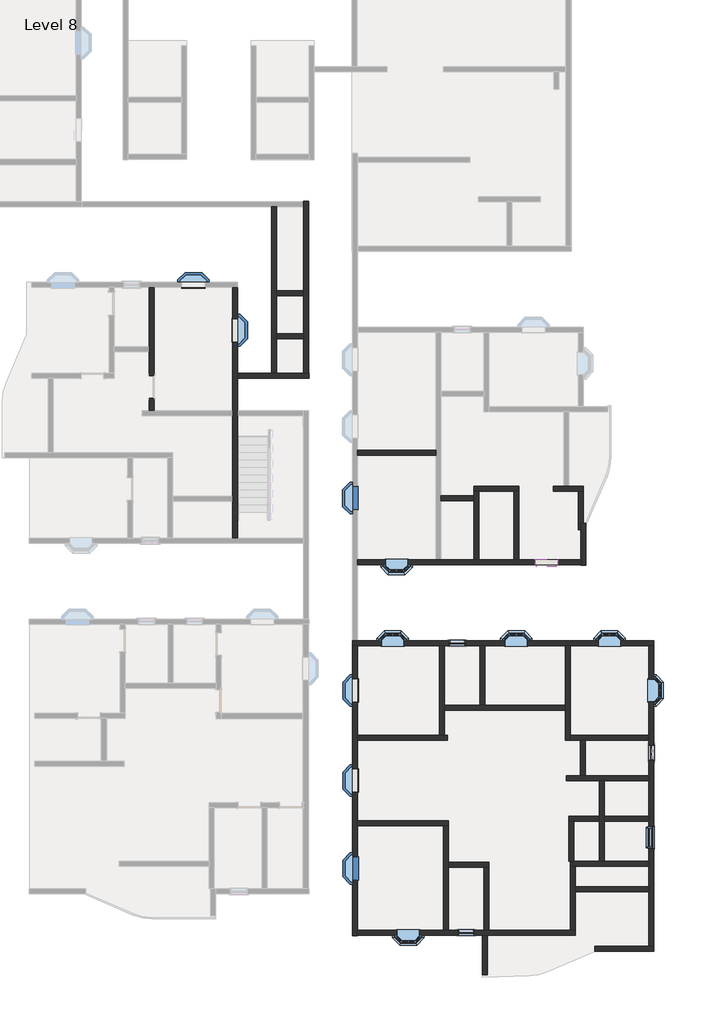
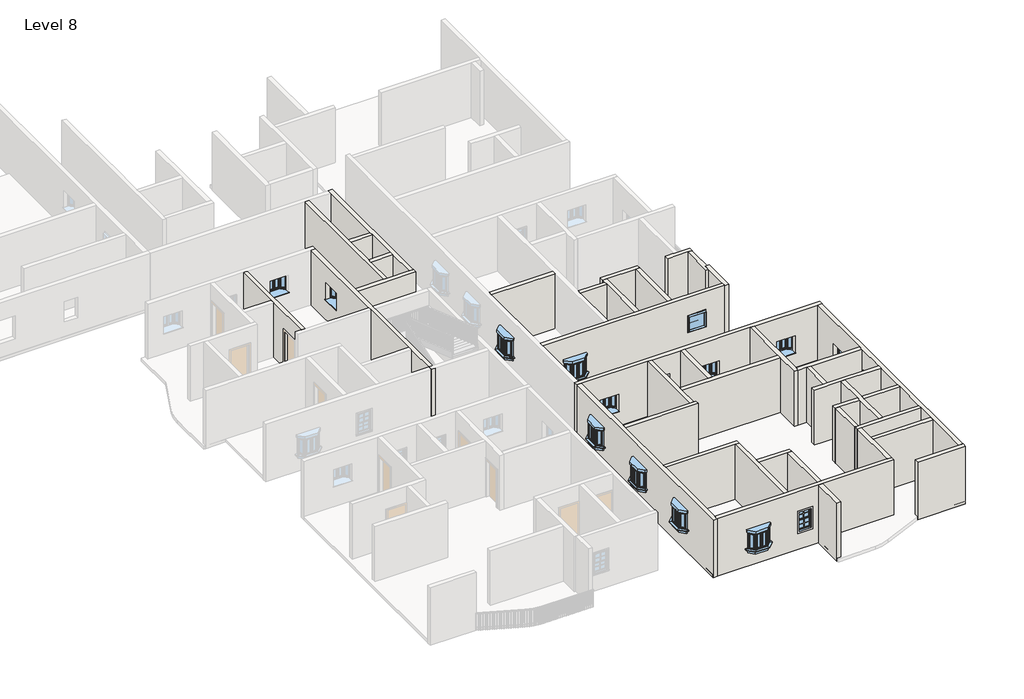
# One storey, part 2 of 14: 40 walls, 17 windows.
"""IFC4 building model written with IfcOpenShell, lengths in millimetres."""

from ifc_helpers import new_model, si_unit, frame, origin, place, context, project, spatial, polyline, outline, extrude, faceted_brep, transform, mapped, element, save
from components import window_910x910mm_67ef725a, window_8debb0fa, windows_sgl_w_glazing_bars_910x910mm_256712d0

model = new_model("IFC4")

# Units and contexts
model_context = context("Model", 3, world=origin())
ifc_project = project(units=[si_unit("LENGTHUNIT", "METRE", prefix="MILLI")], contexts=[model_context])

# Site, building, storey
site = spatial("IfcSite", under=ifc_project)
building = spatial("IfcBuilding", under=site)
storey = spatial("IfcBuildingStorey", under=building, Name="Level 8", Elevation=21336.0)

# Walls
placement = place(None, origin())
element("IfcWall", 1, ObjectType="4.5\" p", at=placement, inside=storey, context=model_context, shape_type="SweptSolid", body=[
    extrude(outline(polyline([(6070.4380523, -28382.7374148), (6070.4380523, -26796.6042694), (6273.6380523, -26796.6042694), (6273.6380523, -28382.7374148), (6070.4380523, -28382.7374148)])), frame((0.0, 0.0, 21336.0), z_axis=(0.0, 0.0, 1.0), x_axis=(1.0, 0.0, 0.0)), (0.0, 0.0, 1.0), 3048.0),
])
element("IfcWall", 2, ObjectType="4.5\" p", at=placement, inside=storey, context=model_context, shape_type="Brep", body=[
    faceted_brep([(10639.6896214, -27431.6042694, 21336.0), (13030.0380523, -27431.6042694, 21336.0), (13030.0380523, -27431.6042694, 24384.0), (10639.6896214, -27431.6042694, 24384.0), (10639.6896214, -27228.4042694, 21336.0), (10639.6896214, -27228.4042694, 24384.0), (12814.1380523, -27228.4042694, 24384.0), (13017.3380523, -27228.4042694, 24384.0), (13030.0380523, -27228.4042694, 24384.0), (13030.0380523, -27228.4042694, 21336.0), (13017.3380523, -27228.4042694, 21336.0), (12814.1380523, -27228.4042694, 21336.0)], [[[0, 1, 2, 3]], [[4, 5, 6, 7, 8, 9, 10, 11]], [[1, 0, 4, 11, 10, 9]], [[2, 1, 9, 8]], [[3, 2, 8, 7, 6, 5]], [[0, 3, 5, 4]]]),
])
element("IfcWall", 3, ObjectType="4.5\" p", at=placement, inside=storey, context=model_context, shape_type="Brep", body=[
    faceted_brep([(1015.8380523, -18878.1542694, 21336.0), (4648.0380523, -18878.1542694, 21336.0), (4648.0380523, -18878.1542694, 24384.0), (1015.8380523, -18878.1542694, 24384.0), (1015.8380523, -18674.9542694, 21336.0), (1015.8380523, -18674.9542694, 24384.0), (4336.8880523, -18674.9542694, 24384.0), (4540.0880523, -18674.9542694, 24384.0), (4648.0380523, -18674.9542694, 24384.0), (4648.0380523, -18674.9542694, 21336.0), (4540.0880523, -18674.9542694, 21336.0), (4336.8880523, -18674.9542694, 21336.0)], [[[0, 1, 2, 3]], [[4, 5, 6, 7, 8, 9, 10, 11]], [[1, 0, 4, 11, 10, 9]], [[2, 1, 9, 8]], [[3, 2, 8, 7, 6, 5]], [[0, 3, 5, 4]]]),
])
element("IfcWall", 4, ObjectType="4.5\" p", at=placement, inside=storey, context=model_context, shape_type="Brep", body=[
    faceted_brep([(4336.8880523, -15049.1042694, 21336.0), (4336.8880523, -18674.9542694, 21336.0), (4336.8880523, -18674.9542694, 24384.0), (4336.8880523, -15049.1042694, 24384.0), (4540.0880523, -15049.1042694, 21336.0), (4540.0880523, -15049.1042694, 24384.0), (4540.0880523, -17455.7542694, 24384.0), (4540.0880523, -17658.9542694, 24384.0), (4540.0880523, -18674.9542694, 24384.0), (4540.0880523, -18674.9542694, 21336.0), (4540.0880523, -17658.9542694, 21336.0), (4540.0880523, -17455.7542694, 21336.0)], [[[0, 1, 2, 3]], [[4, 5, 6, 7, 8, 9, 10, 11]], [[1, 0, 4, 11, 10, 9]], [[3, 2, 8, 7, 6, 5]], [[0, 3, 5, 4]], [[2, 1, 9, 8]]]),
])
element("IfcWall", 5, ObjectType="4.5\" p", at=placement, inside=storey, context=model_context, shape_type="Brep", body=[
    faceted_brep([(4540.0880523, -17658.9542694, 21336.0), (9442.2880523, -17658.9542694, 21336.0), (9442.2880523, -17658.9542694, 24384.0), (4540.0880523, -17658.9542694, 24384.0), (4540.0880523, -17455.7542694, 21336.0), (4540.0880523, -17455.7542694, 24384.0), (5975.1880523, -17455.7542694, 24384.0), (6178.3880523, -17455.7542694, 24384.0), (9442.2880523, -17455.7542694, 24384.0), (9442.2880523, -17455.7542694, 21336.0), (6178.3880523, -17455.7542694, 21336.0), (5975.1880523, -17455.7542694, 21336.0)], [[[0, 1, 2, 3]], [[4, 5, 6, 7, 8, 9, 10, 11]], [[1, 0, 4, 11, 10, 9]], [[3, 2, 8, 7, 6, 5]], [[0, 3, 5, 4]], [[2, 1, 9, 8]]]),
])
element("IfcWall", 6, ObjectType="4.5\" p", at=placement, inside=storey, context=model_context, shape_type="SweptSolid", body=[
    extrude(outline(polyline([(5975.1880523, -17455.7542694), (5975.1880523, -15049.1042694), (6178.3880523, -15049.1042694), (6178.3880523, -17455.7542694), (5975.1880523, -17455.7542694)])), frame((0.0, 0.0, 21336.0), z_axis=(0.0, 0.0, 1.0), x_axis=(1.0, 0.0, 0.0)), (0.0, 0.0, 1.0), 3048.0),
])
element("IfcWall", 7, ObjectType="4.5\" p", at=placement, inside=storey, context=model_context, shape_type="Brep", body=[
    faceted_brep([(9442.2880523, -15049.1042694, 21336.0), (9442.2880523, -17455.7542694, 21336.0), (9442.2880523, -17658.9542694, 21336.0), (9442.2880523, -18871.8042694, 21336.0), (9442.2880523, -18871.8042694, 24384.0), (9442.2880523, -17658.9542694, 24384.0), (9442.2880523, -17455.7542694, 24384.0), (9442.2880523, -15049.1042694, 24384.0), (9645.4880523, -15049.1042694, 21336.0), (9645.4880523, -15049.1042694, 24384.0), (9645.4880523, -18668.6042694, 24384.0), (9645.4880523, -18871.8042694, 24384.0), (9645.4880523, -18871.8042694, 21336.0), (9645.4880523, -18668.6042694, 21336.0)], [[[0, 1, 2, 3, 4, 5, 6, 7]], [[8, 9, 10, 11, 12, 13]], [[3, 2, 1, 0, 8, 13, 12]], [[7, 6, 5, 4, 11, 10, 9]], [[0, 7, 9, 8]], [[4, 3, 12, 11]]]),
])
element("IfcWall", 8, ObjectType="4.5\" p", at=placement, inside=storey, context=model_context, shape_type="Brep", body=[
    faceted_brep([(1015.8380523, -22345.2542694, 21336.0), (4489.2880523, -22345.2542694, 21336.0), (4692.4880523, -22345.2542694, 21336.0), (4692.4880523, -22345.2542694, 24384.0), (4489.2880523, -22345.2542694, 24384.0), (1015.8380523, -22345.2542694, 24384.0), (1015.8380523, -22142.0542694, 21336.0), (1015.8380523, -22142.0542694, 24384.0), (4692.4880523, -22142.0542694, 24384.0), (4692.4880523, -22142.0542694, 21336.0)], [[[0, 1, 2, 3, 4, 5]], [[6, 7, 8, 9]], [[2, 1, 0, 6, 9]], [[5, 4, 3, 8, 7]], [[0, 5, 7, 6]], [[3, 2, 9, 8]]]),
])
element("IfcWall", 9, ObjectType="4.5\" p", at=placement, inside=storey, context=model_context, shape_type="Brep", body=[
    faceted_brep([(4489.2880523, -22345.2542694, 21336.0), (4489.2880523, -26580.7042694, 21336.0), (4489.2880523, -26580.7042694, 24384.0), (4489.2880523, -22345.2542694, 24384.0), (4692.4880523, -22345.2542694, 21336.0), (4692.4880523, -22345.2542694, 24384.0), (4692.4880523, -23818.4542694, 24384.0), (4692.4880523, -24021.6542694, 24384.0), (4692.4880523, -26580.7042694, 24384.0), (4692.4880523, -26580.7042694, 21336.0), (4692.4880523, -24021.6542694, 21336.0), (4692.4880523, -23818.4542694, 21336.0)], [[[0, 1, 2, 3]], [[4, 5, 6, 7, 8, 9, 10, 11]], [[1, 0, 4, 11, 10, 9]], [[3, 2, 8, 7, 6, 5]], [[0, 3, 5, 4]], [[2, 1, 9, 8]]]),
])
element("IfcWall", 10, ObjectType="4.5\" p", at=placement, inside=storey, context=model_context, shape_type="Brep", body=[
    faceted_brep([(4692.4880523, -24021.6542694, 21336.0), (6127.5880523, -24021.6542694, 21336.0), (6330.7880523, -24021.6542694, 21336.0), (6330.7880523, -24021.6542694, 24384.0), (6127.5880523, -24021.6542694, 24384.0), (4692.4880523, -24021.6542694, 24384.0), (4692.4880523, -23818.4542694, 21336.0), (4692.4880523, -23818.4542694, 24384.0), (6330.7880523, -23818.4542694, 24384.0), (6330.7880523, -23818.4542694, 21336.0)], [[[0, 1, 2, 3, 4, 5]], [[6, 7, 8, 9]], [[2, 1, 0, 6, 9]], [[5, 4, 3, 8, 7]], [[0, 5, 7, 6]], [[3, 2, 9, 8]]]),
])
element("IfcWall", 11, ObjectType="4.5\" p", at=placement, inside=storey, context=model_context, shape_type="SweptSolid", body=[
    extrude(outline(polyline([(6127.5880523, -26580.7042694), (6127.5880523, -24021.6542694), (6330.7880523, -24021.6542694), (6330.7880523, -26580.7042694), (6127.5880523, -26580.7042694)])), frame((0.0, 0.0, 21336.0), z_axis=(0.0, 0.0, 1.0), x_axis=(1.0, 0.0, 0.0)), (0.0, 0.0, 1.0), 3048.0),
])
element("IfcWall", 12, ObjectType="4.5\" p", at=placement, inside=storey, context=model_context, shape_type="Brep", body=[
    faceted_brep([(9645.4880523, -18871.8042694, 21336.0), (10051.8880523, -18871.8042694, 21336.0), (10255.0880523, -18871.8042694, 21336.0), (12814.1380523, -18871.8042694, 21336.0), (12814.1380523, -18871.8042694, 24384.0), (10255.0880523, -18871.8042694, 24384.0), (10051.8880523, -18871.8042694, 24384.0), (9645.4880523, -18871.8042694, 24384.0), (9645.4880523, -18668.6042694, 21336.0), (9645.4880523, -18668.6042694, 24384.0), (12814.1380523, -18668.6042694, 24384.0), (12814.1380523, -18668.6042694, 21336.0)], [[[0, 1, 2, 3, 4, 5, 6, 7]], [[8, 9, 10, 11]], [[3, 2, 1, 0, 8, 11]], [[7, 6, 5, 4, 10, 9]], [[0, 7, 9, 8]], [[4, 3, 11, 10]]]),
])
element("IfcWall", 13, ObjectType="4.5\" p", at=placement, inside=storey, context=model_context, shape_type="SweptSolid", body=[
    extrude(outline(polyline([(10051.8880523, -20313.2542694), (10051.8880523, -18871.8042694), (10255.0880523, -18871.8042694), (10255.0880523, -20313.2542694), (10051.8880523, -20313.2542694)])), frame((0.0, 0.0, 21336.0), z_axis=(0.0, 0.0, 1.0), x_axis=(1.0, 0.0, 0.0)), (0.0, 0.0, 1.0), 3048.0),
])
element("IfcWall", 14, ObjectType="4.5\" p", at=placement, inside=storey, context=model_context, shape_type="Brep", body=[
    faceted_brep([(12814.1380523, -20313.2542694, 21336.0), (10255.0880523, -20313.2542694, 21336.0), (10051.8880523, -20313.2542694, 21336.0), (9486.7380523, -20313.2542694, 21336.0), (9486.7380523, -20313.2542694, 24384.0), (10051.8880523, -20313.2542694, 24384.0), (10255.0880523, -20313.2542694, 24384.0), (12814.1380523, -20313.2542694, 24384.0), (12814.1380523, -20516.4542694, 21336.0), (12814.1380523, -20516.4542694, 24384.0), (11017.0880523, -20516.4542694, 24384.0), (10813.8880523, -20516.4542694, 24384.0), (9486.7380523, -20516.4542694, 24384.0), (9486.7380523, -20516.4542694, 21336.0), (10813.8880523, -20516.4542694, 21336.0), (11017.0880523, -20516.4542694, 21336.0)], [[[0, 1, 2, 3, 4, 5, 6, 7]], [[8, 9, 10, 11, 12, 13, 14, 15]], [[3, 2, 1, 0, 8, 15, 14, 13]], [[4, 3, 13, 12]], [[7, 6, 5, 4, 12, 11, 10, 9]], [[0, 7, 9, 8]]]),
])
element("IfcWall", 15, ObjectType="4.5\" p", at=placement, inside=storey, context=model_context, shape_type="Brep", body=[
    faceted_brep([(10813.8880523, -20516.4542694, 21336.0), (10813.8880523, -21951.5542694, 21336.0), (10813.8880523, -22154.7542694, 21336.0), (10813.8880523, -23779.5416506, 21336.0), (10813.8880523, -23779.5416506, 24384.0), (10813.8880523, -22154.7542694, 24384.0), (10813.8880523, -21951.5542694, 24384.0), (10813.8880523, -20516.4542694, 24384.0), (11017.0880523, -20516.4542694, 21336.0), (11017.0880523, -20516.4542694, 24384.0), (11017.0880523, -21951.5542694, 24384.0), (11017.0880523, -22154.7542694, 24384.0), (11017.0880523, -23779.5416506, 24384.0), (11017.0880523, -23779.5416506, 21336.0), (11017.0880523, -22154.7542694, 21336.0), (11017.0880523, -21951.5542694, 21336.0)], [[[0, 1, 2, 3, 4, 5, 6, 7]], [[8, 9, 10, 11, 12, 13, 14, 15]], [[3, 2, 1, 0, 8, 15, 14, 13]], [[7, 6, 5, 4, 12, 11, 10, 9]], [[0, 7, 9, 8]], [[4, 3, 13, 12]]]),
])
element("IfcWall", 16, ObjectType="4.5\" p", at=placement, inside=storey, context=model_context, shape_type="Brep", body=[
    faceted_brep([(12814.1380523, -23779.5416506, 21336.0), (11017.0880523, -23779.5416506, 21336.0), (10813.8880523, -23779.5416506, 21336.0), (9791.5380523, -23779.5416506, 21336.0), (9632.7880523, -23779.5416506, 21336.0), (9632.7880523, -23779.5416506, 24384.0), (9791.5380523, -23779.5416506, 24384.0), (10813.8880523, -23779.5416506, 24384.0), (11017.0880523, -23779.5416506, 24384.0), (12814.1380523, -23779.5416506, 24384.0), (12814.1380523, -23982.7416506, 21336.0), (12814.1380523, -23982.7416506, 24384.0), (9835.9880523, -23982.7416506, 24384.0), (9632.7880523, -23982.7416506, 24384.0), (9632.7880523, -23982.7416506, 21336.0), (9835.9880523, -23982.7416506, 21336.0)], [[[0, 1, 2, 3, 4, 5, 6, 7, 8, 9]], [[10, 11, 12, 13, 14, 15]], [[4, 3, 2, 1, 0, 10, 15, 14]], [[9, 8, 7, 6, 5, 13, 12, 11]], [[0, 9, 11, 10]], [[5, 4, 14, 13]]]),
])
element("IfcWall", 17, ObjectType="4.5\" p", at=placement, inside=storey, context=model_context, shape_type="Brep", body=[
    faceted_brep([(9632.7880523, -23982.7416506, 21336.0), (9632.7880523, -26580.7042694, 21336.0), (9632.7880523, -26580.7042694, 24384.0), (9632.7880523, -23982.7416506, 24384.0), (9835.9880523, -23982.7416506, 21336.0), (9835.9880523, -23982.7416506, 24384.0), (9835.9880523, -24805.3496998, 24384.0), (9835.9880523, -25008.5496998, 24384.0), (9835.9880523, -26580.7042694, 24384.0), (9835.9880523, -26580.7042694, 21336.0), (9835.9880523, -25008.5496998, 21336.0), (9835.9880523, -24805.3496998, 21336.0)], [[[0, 1, 2, 3]], [[4, 5, 6, 7, 8, 9, 10, 11]], [[1, 0, 4, 11, 10, 9]], [[3, 2, 8, 7, 6, 5]], [[2, 1, 9, 8]], [[0, 3, 5, 4]]]),
])
element("IfcWall", 18, ObjectType="4.5\" p", at=placement, inside=storey, context=model_context, shape_type="SweptSolid", body=[
    extrude(outline(polyline([(12814.1380523, -25008.5496998), (9835.9880523, -25008.5496998), (9835.9880523, -24805.3496998), (12814.1380523, -24805.3496998), (12814.1380523, -25008.5496998)])), frame((0.0, 0.0, 21336.0), z_axis=(0.0, 0.0, 1.0), x_axis=(1.0, 0.0, 0.0)), (0.0, 0.0, 1.0), 3048.0),
])
element("IfcWall", 19, ObjectType="4.5\" p", at=placement, inside=storey, context=model_context, shape_type="Brep", body=[
    faceted_brep([(-7432.737215, -5015.2916506, 23469.6), (-7432.737215, -5015.2916506, 21336.0), (-7432.737215, -5523.2916506, 21336.0), (-7432.737215, -5523.2916506, 24384.0), (-7432.737215, -3135.6916506, 24384.0), (-7432.737215, -2932.4916506, 24384.0), (-7432.737215, -525.8416506, 24384.0), (-7432.737215, -525.8416506, 21336.0), (-7432.737215, -2932.4916506, 21336.0), (-7432.737215, -3135.6916506, 21336.0), (-7432.737215, -4100.8916506, 21336.0), (-7432.737215, -4100.8916506, 23469.6), (-7229.537215, -5523.2916506, 21336.0), (-7229.537215, -5015.2916506, 21336.0), (-7229.537215, -5015.2916506, 23469.6), (-7229.537215, -4100.8916506, 23469.6), (-7229.537215, -4100.8916506, 21336.0), (-7229.537215, -525.8416506, 21336.0), (-7229.537215, -525.8416506, 24384.0), (-7229.537215, -5523.2916506, 24384.0)], [[[0, 1, 2, 3, 4, 5, 6, 7, 8, 9, 10, 11]], [[12, 13, 14, 15, 16, 17, 18, 19]], [[2, 1, 13, 12]], [[10, 9, 8, 7, 17, 16]], [[6, 5, 4, 3, 19, 18]], [[7, 6, 18, 17]], [[3, 2, 12, 19]], [[14, 13, 1, 0]], [[15, 14, 0, 11]], [[16, 15, 11, 10]]]),
])
element("IfcWall", 20, ObjectType="4.5\" p", at=placement, inside=storey, context=model_context, shape_type="Brep", body=[
    faceted_brep([(-3857.687215, -4202.4916506, 21336.0), (-961.4891351, -4202.4916506, 21336.0), (-961.4891351, -4202.4916506, 24384.0), (-3857.687215, -4202.4916506, 24384.0), (-3857.687215, -3999.2916506, 21336.0), (-3857.687215, -3999.2916506, 24384.0), (-2472.7891351, -3999.2916506, 24384.0), (-2269.5891351, -3999.2916506, 24384.0), (-1177.3891351, -3999.2916506, 24384.0), (-974.1891351, -3999.2916506, 24384.0), (-961.4891351, -3999.2916506, 24384.0), (-961.4891351, -3999.2916506, 21336.0), (-974.1891351, -3999.2916506, 21336.0), (-1177.3891351, -3999.2916506, 21336.0), (-2269.5891351, -3999.2916506, 21336.0), (-2472.7891351, -3999.2916506, 21336.0)], [[[0, 1, 2, 3]], [[4, 5, 6, 7, 8, 9, 10, 11, 12, 13, 14, 15]], [[1, 0, 4, 15, 14, 13, 12, 11]], [[2, 1, 11, 10]], [[3, 2, 10, 9, 8, 7, 6, 5]], [[0, 3, 5, 4]]]),
])
element("IfcWall", 21, ObjectType="4.5\" p", at=placement, inside=storey, context=model_context, shape_type="SweptSolid", body=[
    extrude(outline(polyline([(-1177.3891351, -868.7416506), (-2269.5891351, -868.7416506), (-2269.5891351, -665.5416506), (-1177.3891351, -665.5416506), (-1177.3891351, -868.7416506)])), frame((0.0, 0.0, 21336.0), z_axis=(0.0, 0.0, 1.0), x_axis=(1.0, 0.0, 0.0)), (0.0, 0.0, 1.0), 3048.0),
])
element("IfcWall", 22, ObjectType="4.5\" p", at=placement, inside=storey, context=model_context, shape_type="SweptSolid", body=[
    extrude(outline(polyline([(-1177.3891351, -2597.8466506), (-2269.5891351, -2597.8466506), (-2269.5891351, -2394.6466506), (-1177.3891351, -2394.6466506), (-1177.3891351, -2597.8466506)])), frame((0.0, 0.0, 21336.0), z_axis=(0.0, 0.0, 1.0), x_axis=(1.0, 0.0, 0.0)), (0.0, 0.0, 1.0), 3048.0),
])
element("IfcWall", 23, ObjectType="4.5\" p", at=placement, inside=storey, context=model_context, shape_type="SweptSolid", body=[
    extrude(outline(polyline([(5721.1880523, -9162.6542694), (4387.6880523, -9162.6542694), (4387.6880523, -8959.4542694), (5721.1880523, -8959.4542694), (5721.1880523, -9162.6542694)])), frame((0.0, 0.0, 21336.0), z_axis=(0.0, 0.0, 1.0), x_axis=(1.0, 0.0, 0.0)), (0.0, 0.0, 1.0), 3048.0),
])
element("IfcWall", 24, ObjectType="4.5\" p", at=placement, inside=storey, context=model_context, shape_type="Brep", body=[
    faceted_brep([(5721.1880523, -8781.6542694, 21336.0), (5924.3880523, -8781.6542694, 21336.0), (7359.4880523, -8781.6542694, 21336.0), (7562.6880523, -8781.6542694, 21336.0), (7562.6880523, -8781.6542694, 24384.0), (7359.4880523, -8781.6542694, 24384.0), (5924.3880523, -8781.6542694, 24384.0), (5721.1880523, -8781.6542694, 24384.0), (5721.1880523, -8578.4542694, 21336.0), (5721.1880523, -8578.4542694, 24384.0), (7562.6880523, -8578.4542694, 24384.0), (7562.6880523, -8578.4542694, 21336.0)], [[[0, 1, 2, 3, 4, 5, 6, 7]], [[8, 9, 10, 11]], [[3, 2, 1, 0, 8, 11]], [[7, 6, 5, 4, 10, 9]], [[0, 7, 9, 8]], [[4, 3, 11, 10]]]),
])
element("IfcWall", 25, ObjectType="4.5\" p", at=placement, inside=storey, context=model_context, shape_type="Brep", body=[
    faceted_brep([(5721.1880523, -8781.6542694, 21336.0), (5721.1880523, -8959.4542694, 21336.0), (5721.1880523, -9162.6542694, 21336.0), (5721.1880523, -11556.6042694, 21336.0), (5721.1880523, -11556.6042694, 24384.0), (5721.1880523, -9162.6542694, 24384.0), (5721.1880523, -8959.4542694, 24384.0), (5721.1880523, -8781.6542694, 24384.0), (5924.3880523, -8781.6542694, 21336.0), (5924.3880523, -8781.6542694, 24384.0), (5924.3880523, -11556.6042694, 24384.0), (5924.3880523, -11556.6042694, 21336.0)], [[[0, 1, 2, 3, 4, 5, 6, 7]], [[8, 9, 10, 11]], [[3, 2, 1, 0, 8, 11]], [[7, 6, 5, 4, 10, 9]], [[0, 7, 9, 8]], [[4, 3, 11, 10]]]),
])
element("IfcWall", 26, ObjectType="4.5\" p", at=placement, inside=storey, context=model_context, shape_type="SweptSolid", body=[
    extrude(outline(polyline([(7359.4880523, -11556.6042694), (7359.4880523, -8781.6542694), (7562.6880523, -8781.6542694), (7562.6880523, -11556.6042694), (7359.4880523, -11556.6042694)])), frame((0.0, 0.0, 21336.0), z_axis=(0.0, 0.0, 1.0), x_axis=(1.0, 0.0, 0.0)), (0.0, 0.0, 1.0), 3048.0),
])
element("IfcWall", 27, ObjectType="4.5\" p", at=placement, inside=storey, context=model_context, shape_type="SweptSolid", body=[
    extrude(outline(polyline([(4184.4880523, -7333.8542694), (1007.0108649, -7333.8542694), (1007.0108649, -7130.6542694), (4184.4880523, -7130.6542694), (4184.4880523, -7333.8542694)])), frame((0.0, 0.0, 21336.0), z_axis=(0.0, 0.0, 1.0), x_axis=(1.0, 0.0, 0.0)), (0.0, 0.0, 1.0), 3048.0),
])
element("IfcWall", 28, ObjectType="4.5\" p", at=placement, inside=storey, context=model_context, shape_type="Brep", body=[
    faceted_brep([(8953.3380523, -8781.6542694, 21336.0), (9956.6380523, -8781.6542694, 21336.0), (10159.8380523, -8781.6542694, 21336.0), (10172.5380523, -8781.6542694, 21336.0), (10172.5380523, -8781.6542694, 24384.0), (10159.8380523, -8781.6542694, 24384.0), (9956.6380523, -8781.6542694, 24384.0), (8953.3380523, -8781.6542694, 24384.0), (8953.3380523, -8578.4542694, 21336.0), (8953.3380523, -8578.4542694, 24384.0), (9371.2322031, -8578.4542694, 24384.0), (9574.4322031, -8578.4542694, 24384.0), (10172.5380523, -8578.4542694, 24384.0), (10172.5380523, -8578.4542694, 21336.0), (9574.4322031, -8578.4542694, 21336.0), (9371.2322031, -8578.4542694, 21336.0)], [[[0, 1, 2, 3, 4, 5, 6, 7]], [[8, 9, 10, 11, 12, 13, 14, 15]], [[3, 2, 1, 0, 8, 15, 14, 13]], [[4, 3, 13, 12]], [[7, 6, 5, 4, 12, 11, 10, 9]], [[0, 7, 9, 8]]]),
])
element("IfcWall", 29, ObjectType="4.5\" p", at=placement, inside=storey, context=model_context, shape_type="SweptSolid", body=[
    extrude(outline(polyline([(9956.6380523, -10352.8912671), (9956.6380523, -8781.6542694), (10159.8380523, -8781.6542694), (10159.8380523, -10352.8912671), (9956.6380523, -10352.8912671)])), frame((0.0, 0.0, 21336.0), z_axis=(0.0, 0.0, 1.0), x_axis=(1.0, 0.0, 0.0)), (0.0, 0.0, 1.0), 3048.0),
])
element("IfcWall", 30, ObjectType="4.5\" p", at=placement, inside=storey, context=model_context, shape_type="Brep", body=[
    faceted_brep([(12814.1380523, -21951.5542694, 24384.0), (12814.1380523, -21951.5542694, 21336.0), (11017.0880523, -21951.5542694, 21336.0), (11017.0880523, -21951.5542694, 24384.0), (12814.1380523, -22154.7542694, 21336.0), (12814.1380523, -22154.7542694, 24384.0), (11017.0880523, -22154.7542694, 24384.0), (11017.0880523, -22154.7542694, 21336.0)], [[[0, 1, 2, 3]], [[4, 5, 6, 7]], [[1, 4, 7, 2]], [[5, 0, 3, 6]], [[1, 0, 5, 4]], [[3, 2, 7, 6]]]),
    faceted_brep([(9588.3380523, -21951.5542694, 21336.0), (9588.3380523, -21951.5542694, 24384.0), (10813.8880523, -21951.5542694, 24384.0), (10813.8880523, -21951.5542694, 21336.0), (9588.3380523, -22154.7542694, 24384.0), (9588.3380523, -22154.7542694, 21336.0), (9791.5380523, -22154.7542694, 21336.0), (10813.8880523, -22154.7542694, 21336.0), (10813.8880523, -22154.7542694, 24384.0), (9791.5380523, -22154.7542694, 24384.0)], [[[0, 1, 2, 3]], [[4, 5, 6, 7, 8, 9]], [[5, 0, 3, 7, 6]], [[1, 4, 9, 8, 2]], [[3, 2, 8, 7]], [[1, 0, 5, 4]]]),
])
element("IfcWall", 31, ObjectType="4.5\" p", at=placement, inside=storey, context=model_context, shape_type="Brep", body=[
    faceted_brep([(9588.3380523, -22154.7542694, 21336.0), (9588.3380523, -23779.5416506, 21336.0), (9588.3380523, -23779.5416506, 24384.0), (9588.3380523, -22154.7542694, 24384.0), (9791.5380523, -22154.7542694, 21336.0), (9791.5380523, -22154.7542694, 24384.0), (9791.5380523, -23779.5416506, 24384.0), (9791.5380523, -23779.5416506, 21336.0), (9632.7880523, -23779.5416506, 21336.0), (9632.7880523, -23779.5416506, 24384.0)], [[[0, 1, 2, 3]], [[4, 5, 6, 7]], [[1, 0, 4, 7, 8]], [[3, 2, 9, 6, 5]], [[2, 1, 8, 7, 6, 9]], [[0, 3, 5, 4]]]),
])
element("IfcWall", 32, ObjectType="9\"", at=placement, inside=storey, context=model_context, shape_type="Brep", body=[
    faceted_brep([(799.9380523, -15049.1042694, 21336.0), (812.6380523, -15049.1042694, 21336.0), (1015.8380523, -15049.1042694, 21336.0), (4336.8880523, -15049.1042694, 21336.0), (4540.0880523, -15049.1042694, 21336.0), (5975.1880523, -15049.1042694, 21336.0), (6178.3880523, -15049.1042694, 21336.0), (9442.2880523, -15049.1042694, 21336.0), (9645.4880523, -15049.1042694, 21336.0), (12814.1380523, -15049.1042694, 21336.0), (13017.3380523, -15049.1042694, 21336.0), (13030.0380523, -15049.1042694, 21336.0), (13030.0380523, -15049.1042694, 24384.0), (13017.3380523, -15049.1042694, 24384.0), (12814.1380523, -15049.1042694, 24384.0), (9645.4880523, -15049.1042694, 24384.0), (9442.2880523, -15049.1042694, 24384.0), (6178.3880523, -15049.1042694, 24384.0), (5975.1880523, -15049.1042694, 24384.0), (4540.0880523, -15049.1042694, 24384.0), (4336.8880523, -15049.1042694, 24384.0), (1015.8380523, -15049.1042694, 24384.0), (812.6380523, -15049.1042694, 24384.0), (799.9380523, -15049.1042694, 24384.0), (1983.2380523, -15049.1042694, 23160.4), (2893.2380523, -15049.1042694, 23160.4), (2893.2380523, -15049.1042694, 22250.4), (1983.2380523, -15049.1042694, 22250.4), (10774.8130523, -15049.1042694, 23160.4), (11684.8130523, -15049.1042694, 23160.4), (11684.8130523, -15049.1042694, 22250.4), (10774.8130523, -15049.1042694, 22250.4), (6993.3880523, -15049.1042694, 23160.4), (7903.3880523, -15049.1042694, 23160.4), (7903.3880523, -15049.1042694, 22250.4), (6993.3880523, -15049.1042694, 22250.4), (4717.8880523, -15049.1042694, 23317.2), (5378.2880523, -15049.1042694, 23317.2), (5378.2880523, -15049.1042694, 22250.4), (4717.8880523, -15049.1042694, 22250.4), (799.9380523, -14845.9042694, 21336.0), (799.9380523, -14845.9042694, 24384.0), (803.8108649, -14845.9042694, 24384.0), (1007.0108649, -14845.9042694, 24384.0), (13030.0380523, -14845.9042694, 24384.0), (13030.0380523, -14845.9042694, 21336.0), (1007.0108649, -14845.9042694, 21336.0), (803.8108649, -14845.9042694, 21336.0), (1983.2380523, -14845.9042694, 23160.4), (1983.2380523, -14845.9042694, 22250.4), (2893.2380523, -14845.9042694, 22250.4), (2893.2380523, -14845.9042694, 23160.4), (10774.8130523, -14845.9042694, 23160.4), (10774.8130523, -14845.9042694, 22250.4), (11684.8130523, -14845.9042694, 22250.4), (11684.8130523, -14845.9042694, 23160.4), (6993.3880523, -14845.9042694, 23160.4), (6993.3880523, -14845.9042694, 22250.4), (7903.3880523, -14845.9042694, 22250.4), (7903.3880523, -14845.9042694, 23160.4), (4717.8880523, -14845.9042694, 23317.2), (4717.8880523, -14845.9042694, 22250.4), (5378.2880523, -14845.9042694, 22250.4), (5378.2880523, -14845.9042694, 23317.2)], [[[0, 1, 2, 3, 4, 5, 6, 7, 8, 9, 10, 11, 12, 13, 14, 15, 16, 17, 18, 19, 20, 21, 22, 23], [24, 25, 26, 27], [28, 29, 30, 31], [32, 33, 34, 35], [36, 37, 38, 39]], [[40, 41, 42, 43, 44, 45, 46, 47], [48, 49, 50, 51], [52, 53, 54, 55], [56, 57, 58, 59], [60, 61, 62, 63]], [[11, 10, 9, 8, 7, 6, 5, 4, 3, 2, 1, 0, 40, 47, 46, 45]], [[12, 11, 45, 44]], [[23, 22, 21, 20, 19, 18, 17, 16, 15, 14, 13, 12, 44, 43, 42, 41]], [[0, 23, 41, 40]], [[49, 48, 24, 27]], [[50, 49, 27, 26]], [[51, 50, 26, 25]], [[48, 51, 25, 24]], [[53, 52, 28, 31]], [[54, 53, 31, 30]], [[55, 54, 30, 29]], [[52, 55, 29, 28]], [[57, 56, 32, 35]], [[58, 57, 35, 34]], [[59, 58, 34, 33]], [[56, 59, 33, 32]], [[61, 60, 36, 39]], [[62, 61, 39, 38]], [[63, 62, 38, 37]], [[60, 63, 37, 36]]]),
])
element("IfcWall", 33, ObjectType="9\"", at=placement, inside=storey, context=model_context, shape_type="Brep", body=[
    faceted_brep([(12814.1380523, -15049.1042694, 21336.0), (12814.1380523, -18668.6042694, 21336.0), (12814.1380523, -18871.8042694, 21336.0), (12814.1380523, -20313.2542694, 21336.0), (12814.1380523, -20516.4542694, 21336.0), (12814.1380523, -21951.5542694, 21336.0), (12814.1380523, -22154.7542694, 21336.0), (12814.1380523, -23779.5416506, 21336.0), (12814.1380523, -23982.7416506, 21336.0), (12814.1380523, -24805.3496998, 21336.0), (12814.1380523, -25008.5496998, 21336.0), (12814.1380523, -27228.4042694, 21336.0), (12814.1380523, -27228.4042694, 24384.0), (12814.1380523, -25008.5496998, 24384.0), (12814.1380523, -24805.3496998, 24384.0), (12814.1380523, -23982.7416506, 24384.0), (12814.1380523, -23779.5416506, 24384.0), (12814.1380523, -22154.7542694, 24384.0), (12814.1380523, -21951.5542694, 24384.0), (12814.1380523, -20516.4542694, 24384.0), (12814.1380523, -20313.2542694, 24384.0), (12814.1380523, -18871.8042694, 24384.0), (12814.1380523, -18668.6042694, 24384.0), (12814.1380523, -15049.1042694, 24384.0), (12814.1380523, -16403.8542694, 23160.4), (12814.1380523, -17313.8542694, 23160.4), (12814.1380523, -17313.8542694, 22250.4), (12814.1380523, -16403.8542694, 22250.4), (12814.1380523, -23270.1542694, 23160.4), (12814.1380523, -23270.1542694, 22250.4), (12814.1380523, -22360.1542694, 22250.4), (12814.1380523, -22360.1542694, 23160.4), (12814.1380523, -19049.6042694, 23317.2), (12814.1380523, -19710.0042694, 23317.2), (12814.1380523, -19710.0042694, 22250.4), (12814.1380523, -19049.6042694, 22250.4), (13017.3380523, -15049.1042694, 21336.0), (13017.3380523, -15049.1042694, 24384.0), (13017.3380523, -27228.4042694, 24384.0), (13017.3380523, -27228.4042694, 21336.0), (13017.3380523, -16403.8542694, 23160.4), (13017.3380523, -16403.8542694, 22250.4), (13017.3380523, -17313.8542694, 22250.4), (13017.3380523, -17313.8542694, 23160.4), (13017.3380523, -23270.1542694, 23160.4), (13017.3380523, -22360.1542694, 23160.4), (13017.3380523, -22360.1542694, 22250.4), (13017.3380523, -23270.1542694, 22250.4), (13017.3380523, -19049.6042694, 23317.2), (13017.3380523, -19049.6042694, 22250.4), (13017.3380523, -19710.0042694, 22250.4), (13017.3380523, -19710.0042694, 23317.2)], [[[0, 1, 2, 3, 4, 5, 6, 7, 8, 9, 10, 11, 12, 13, 14, 15, 16, 17, 18, 19, 20, 21, 22, 23], [24, 25, 26, 27], [28, 29, 30, 31], [32, 33, 34, 35]], [[36, 37, 38, 39], [40, 41, 42, 43], [44, 45, 46, 47], [48, 49, 50, 51]], [[11, 10, 9, 8, 7, 6, 5, 4, 3, 2, 1, 0, 36, 39]], [[23, 22, 21, 20, 19, 18, 17, 16, 15, 14, 13, 12, 38, 37]], [[0, 23, 37, 36]], [[12, 11, 39, 38]], [[41, 40, 24, 27]], [[42, 41, 27, 26]], [[43, 42, 26, 25]], [[40, 43, 25, 24]], [[29, 28, 44, 47]], [[30, 29, 47, 46]], [[31, 30, 46, 45]], [[28, 31, 45, 44]], [[49, 48, 32, 35]], [[50, 49, 35, 34]], [[51, 50, 34, 33]], [[48, 51, 33, 32]]]),
])
element("IfcWall", 34, ObjectType="9\"", at=placement, inside=storey, context=model_context, shape_type="Brep", body=[
    faceted_brep([(812.6380523, -15049.1042694, 21336.0), (812.6380523, -26796.6042694, 21336.0), (812.6380523, -26796.6042694, 24384.0), (812.6380523, -15049.1042694, 24384.0), (812.6380523, -24527.4542694, 23446.0), (812.6380523, -24527.4542694, 22536.0), (812.6380523, -23617.4542694, 22536.0), (812.6380523, -23617.4542694, 23446.0), (812.6380523, -20965.1042694, 23446.0), (812.6380523, -20965.1042694, 22536.0), (812.6380523, -20055.1042694, 22536.0), (812.6380523, -20055.1042694, 23446.0), (812.6380523, -17317.0292694, 23446.0), (812.6380523, -17317.0292694, 22536.0), (812.6380523, -16407.0292694, 22536.0), (812.6380523, -16407.0292694, 23446.0), (1015.8380523, -15049.1042694, 21336.0), (1015.8380523, -15049.1042694, 24384.0), (1015.8380523, -18674.9542694, 24384.0), (1015.8380523, -18878.1542694, 24384.0), (1015.8380523, -22142.0542694, 24384.0), (1015.8380523, -22345.2542694, 24384.0), (1015.8380523, -26580.7042694, 24384.0), (1015.8380523, -26783.9042694, 24384.0), (1015.8380523, -26796.6042694, 24384.0), (1015.8380523, -26796.6042694, 21336.0), (1015.8380523, -26783.9042694, 21336.0), (1015.8380523, -26580.7042694, 21336.0), (1015.8380523, -22345.2542694, 21336.0), (1015.8380523, -22142.0542694, 21336.0), (1015.8380523, -18878.1542694, 21336.0), (1015.8380523, -18674.9542694, 21336.0), (1015.8380523, -24527.4542694, 23446.0), (1015.8380523, -23617.4542694, 23446.0), (1015.8380523, -23617.4542694, 22536.0), (1015.8380523, -24527.4542694, 22536.0), (1015.8380523, -20965.1042694, 23446.0), (1015.8380523, -20055.1042694, 23446.0), (1015.8380523, -20055.1042694, 22536.0), (1015.8380523, -20965.1042694, 22536.0), (1015.8380523, -17317.0292694, 23446.0), (1015.8380523, -16407.0292694, 23446.0), (1015.8380523, -16407.0292694, 22536.0), (1015.8380523, -17317.0292694, 22536.0)], [[[0, 1, 2, 3], [4, 5, 6, 7], [8, 9, 10, 11], [12, 13, 14, 15]], [[16, 17, 18, 19, 20, 21, 22, 23, 24, 25, 26, 27, 28, 29, 30, 31], [32, 33, 34, 35], [36, 37, 38, 39], [40, 41, 42, 43]], [[1, 0, 16, 31, 30, 29, 28, 27, 26, 25]], [[2, 1, 25, 24]], [[3, 2, 24, 23, 22, 21, 20, 19, 18, 17]], [[0, 3, 17, 16]], [[5, 4, 32, 35]], [[6, 5, 35, 34]], [[7, 6, 34, 33]], [[4, 7, 33, 32]], [[9, 8, 36, 39]], [[10, 9, 39, 38]], [[11, 10, 38, 37]], [[8, 11, 37, 36]], [[13, 12, 40, 43]], [[14, 13, 43, 42]], [[15, 14, 42, 41]], [[12, 15, 41, 40]]]),
])
element("IfcWall", 35, ObjectType="9\"", at=placement, inside=storey, context=model_context, shape_type="Brep", body=[
    faceted_brep([(1015.8380523, -26783.9042694, 21336.0), (9835.9880523, -26783.9042694, 21336.0), (9835.9880523, -26783.9042694, 24384.0), (1015.8380523, -26783.9042694, 24384.0), (3521.8880523, -26783.9042694, 23160.4), (3521.8880523, -26783.9042694, 22250.4), (2611.8880523, -26783.9042694, 22250.4), (2611.8880523, -26783.9042694, 23160.4), (5079.8380523, -26783.9042694, 23317.2), (5740.2380523, -26783.9042694, 23317.2), (5740.2380523, -26783.9042694, 22250.4), (5079.8380523, -26783.9042694, 22250.4), (1015.8380523, -26580.7042694, 21336.0), (1015.8380523, -26580.7042694, 24384.0), (4489.2880523, -26580.7042694, 24384.0), (4692.4880523, -26580.7042694, 24384.0), (6127.5880523, -26580.7042694, 24384.0), (6330.7880523, -26580.7042694, 24384.0), (9632.7880523, -26580.7042694, 24384.0), (9835.9880523, -26580.7042694, 24384.0), (9835.9880523, -26580.7042694, 21336.0), (9632.7880523, -26580.7042694, 21336.0), (6330.7880523, -26580.7042694, 21336.0), (6127.5880523, -26580.7042694, 21336.0), (4692.4880523, -26580.7042694, 21336.0), (4489.2880523, -26580.7042694, 21336.0), (3521.8880523, -26580.7042694, 23160.4), (2611.8880523, -26580.7042694, 23160.4), (2611.8880523, -26580.7042694, 22250.4), (3521.8880523, -26580.7042694, 22250.4), (5079.8380523, -26580.7042694, 23317.2), (5079.8380523, -26580.7042694, 22250.4), (5740.2380523, -26580.7042694, 22250.4), (5740.2380523, -26580.7042694, 23317.2)], [[[0, 1, 2, 3], [4, 5, 6, 7], [8, 9, 10, 11]], [[12, 13, 14, 15, 16, 17, 18, 19, 20, 21, 22, 23, 24, 25], [26, 27, 28, 29], [30, 31, 32, 33]], [[1, 0, 12, 25, 24, 23, 22, 21, 20]], [[3, 2, 19, 18, 17, 16, 15, 14, 13]], [[0, 3, 13, 12]], [[2, 1, 20, 19]], [[5, 4, 26, 29]], [[6, 5, 29, 28]], [[7, 6, 28, 27]], [[4, 7, 27, 26]], [[31, 30, 8, 11]], [[32, 31, 11, 10]], [[33, 32, 10, 9]], [[30, 33, 9, 8]]]),
])
element("IfcWall", 36, ObjectType="9\" w", at=placement, inside=storey, context=model_context, shape_type="Brep", body=[
    faceted_brep([(-4060.887215, -525.8416506, 21336.0), (-4060.887215, -5523.2916506, 21336.0), (-4060.887215, -5726.4916506, 21336.0), (-4060.887215, -8990.3916506, 21336.0), (-4060.887215, -9193.5916506, 21336.0), (-4060.887215, -10901.7416506, 21336.0), (-4060.887215, -10901.7416506, 24384.0), (-4060.887215, -9193.5916506, 24384.0), (-4060.887215, -8990.3916506, 24384.0), (-4060.887215, -5726.4916506, 24384.0), (-4060.887215, -5523.2916506, 24384.0), (-4060.887215, -525.8416506, 24384.0), (-4060.887215, -1807.5666506, 23446.0), (-4060.887215, -2717.5666506, 23446.0), (-4060.887215, -2717.5666506, 22536.0), (-4060.887215, -1807.5666506, 22536.0), (-3857.687215, -525.8416506, 21336.0), (-3857.687215, -525.8416506, 24384.0), (-3857.687215, -3999.2916506, 24384.0), (-3857.687215, -4202.4916506, 24384.0), (-3857.687215, -5523.2916506, 24384.0), (-3857.687215, -5726.4916506, 24384.0), (-3857.687215, -10901.7416506, 24384.0), (-3857.687215, -10901.7416506, 21336.0), (-3857.687215, -5726.4916506, 21336.0), (-3857.687215, -5523.2916506, 21336.0), (-3857.687215, -4202.4916506, 21336.0), (-3857.687215, -3999.2916506, 21336.0), (-3857.687215, -1807.5666506, 23446.0), (-3857.687215, -1807.5666506, 22536.0), (-3857.687215, -2717.5666506, 22536.0), (-3857.687215, -2717.5666506, 23446.0)], [[[0, 1, 2, 3, 4, 5, 6, 7, 8, 9, 10, 11], [12, 13, 14, 15]], [[16, 17, 18, 19, 20, 21, 22, 23, 24, 25, 26, 27], [28, 29, 30, 31]], [[5, 4, 3, 2, 1, 0, 16, 27, 26, 25, 24, 23]], [[6, 5, 23, 22]], [[11, 10, 9, 8, 7, 6, 22, 21, 20, 19, 18, 17]], [[0, 11, 17, 16]], [[29, 28, 12, 15]], [[30, 29, 15, 14]], [[31, 30, 14, 13]], [[28, 31, 13, 12]]]),
])
element("IfcWall", 37, ObjectType="9\" w", at=placement, inside=storey, context=model_context, shape_type="Brep", body=[
    faceted_brep([(-2269.5891351, -3999.2916506, 21336.0), (-2269.5891351, -2597.8466506, 21336.0), (-2269.5891351, -2394.6466506, 21336.0), (-2269.5891351, -868.7416506, 21336.0), (-2269.5891351, -665.5416506, 21336.0), (-2269.5891351, 2750.7583494, 21336.0), (-2269.5891351, 2750.7583494, 24384.0), (-2269.5891351, -665.5416506, 24384.0), (-2269.5891351, -868.7416506, 24384.0), (-2269.5891351, -2394.6466506, 24384.0), (-2269.5891351, -2597.8466506, 24384.0), (-2269.5891351, -3999.2916506, 24384.0), (-2472.7891351, -3999.2916506, 21336.0), (-2472.7891351, -3999.2916506, 24384.0), (-2472.7891351, 2750.7583494, 24384.0), (-2472.7891351, 2750.7583494, 21336.0)], [[[0, 1, 2, 3, 4, 5, 6, 7, 8, 9, 10, 11]], [[12, 13, 14, 15]], [[5, 4, 3, 2, 1, 0, 12, 15]], [[11, 10, 9, 8, 7, 6, 14, 13]], [[0, 11, 13, 12]], [[6, 5, 15, 14]]]),
])
element("IfcWall", 38, ObjectType="9\" w", at=placement, inside=storey, context=model_context, shape_type="Brep", body=[
    faceted_brep([(-974.1891351, -3999.2916506, 21336.0), (-974.1891351, 2966.6583494, 21336.0), (-974.1891351, 2966.6583494, 24384.0), (-974.1891351, -3999.2916506, 24384.0), (-1177.3891351, -3999.2916506, 21336.0), (-1177.3891351, -3999.2916506, 24384.0), (-1177.3891351, -2597.8466506, 24384.0), (-1177.3891351, -2394.6466506, 24384.0), (-1177.3891351, -868.7416506, 24384.0), (-1177.3891351, -665.5416506, 24384.0), (-1177.3891351, 2750.7583494, 24384.0), (-1177.3891351, 2953.9583494, 24384.0), (-1177.3891351, 2966.6583494, 24384.0), (-1177.3891351, 2966.6583494, 21336.0), (-1177.3891351, 2953.9583494, 21336.0), (-1177.3891351, 2750.7583494, 21336.0), (-1177.3891351, -665.5416506, 21336.0), (-1177.3891351, -868.7416506, 21336.0), (-1177.3891351, -2394.6466506, 21336.0), (-1177.3891351, -2597.8466506, 21336.0)], [[[0, 1, 2, 3]], [[4, 5, 6, 7, 8, 9, 10, 11, 12, 13, 14, 15, 16, 17, 18, 19]], [[1, 0, 4, 19, 18, 17, 16, 15, 14, 13]], [[2, 1, 13, 12]], [[3, 2, 12, 11, 10, 9, 8, 7, 6, 5]], [[0, 3, 5, 4]]]),
])
element("IfcWall", 39, ObjectType="9\" w", at=placement, inside=storey, context=model_context, shape_type="Brep", body=[
    faceted_brep([(1007.0108649, -11759.8042694, 21336.0), (10070.9380523, -11759.8042694, 21336.0), (10070.9380523, -11759.8042694, 24384.0), (1007.0108649, -11759.8042694, 24384.0), (3050.7494586, -11759.8042694, 23160.4), (3050.7494586, -11759.8042694, 22250.4), (2140.7494586, -11759.8042694, 22250.4), (2140.7494586, -11759.8042694, 23160.4), (9135.2880523, -11759.8042694, 23446.0), (9135.2880523, -11759.8042694, 22536.0), (8225.2880523, -11759.8042694, 22536.0), (8225.2880523, -11759.8042694, 23446.0), (1007.0108649, -11556.6042694, 21336.0), (1007.0108649, -11556.6042694, 24384.0), (4184.4880523, -11556.6042694, 24384.0), (4387.6880523, -11556.6042694, 24384.0), (5721.1880523, -11556.6042694, 24384.0), (5924.3880523, -11556.6042694, 24384.0), (7359.4880523, -11556.6042694, 24384.0), (7562.6880523, -11556.6042694, 24384.0), (10070.9380523, -11556.6042694, 24384.0), (10070.9380523, -11556.6042694, 21336.0), (7562.6880523, -11556.6042694, 21336.0), (7359.4880523, -11556.6042694, 21336.0), (5924.3880523, -11556.6042694, 21336.0), (5721.1880523, -11556.6042694, 21336.0), (4387.6880523, -11556.6042694, 21336.0), (4184.4880523, -11556.6042694, 21336.0), (3050.7494586, -11556.6042694, 23160.4), (2140.7494586, -11556.6042694, 23160.4), (2140.7494586, -11556.6042694, 22250.4), (3050.7494586, -11556.6042694, 22250.4), (9135.2880523, -11556.6042694, 23446.0), (8225.2880523, -11556.6042694, 23446.0), (8225.2880523, -11556.6042694, 22536.0), (9135.2880523, -11556.6042694, 22536.0)], [[[0, 1, 2, 3], [4, 5, 6, 7], [8, 9, 10, 11]], [[12, 13, 14, 15, 16, 17, 18, 19, 20, 21, 22, 23, 24, 25, 26, 27], [28, 29, 30, 31], [32, 33, 34, 35]], [[1, 0, 12, 27, 26, 25, 24, 23, 22, 21]], [[3, 2, 20, 19, 18, 17, 16, 15, 14, 13]], [[0, 3, 13, 12]], [[2, 1, 21, 20]], [[5, 4, 28, 31]], [[6, 5, 31, 30]], [[7, 6, 30, 29]], [[4, 7, 29, 28]], [[9, 8, 32, 35]], [[10, 9, 35, 34]], [[11, 10, 34, 33]], [[8, 11, 33, 32]]]),
])
element("IfcWall", 40, ObjectType="9\" w", at=placement, inside=storey, context=model_context, shape_type="Brep", body=[
    faceted_brep([(10070.9380523, -10085.9721442, 21336.0), (10070.9380523, -11556.6042694, 21336.0), (10070.9380523, -11759.8042694, 21336.0), (10070.9380523, -11785.2042694, 21336.0), (10070.9380523, -11785.2042694, 24384.0), (10070.9380523, -11759.8042694, 24384.0), (10070.9380523, -11556.6042694, 24384.0), (10070.9380523, -10085.9721442, 24384.0), (10274.1380523, -10085.9721442, 21336.0), (10274.1380523, -10085.9721442, 24384.0), (10274.1380523, -11785.2042694, 24384.0), (10274.1380523, -11785.2042694, 21336.0)], [[[0, 1, 2, 3, 4, 5, 6, 7]], [[8, 9, 10, 11]], [[3, 2, 1, 0, 8, 11]], [[4, 3, 11, 10]], [[7, 6, 5, 4, 10, 9]], [[0, 7, 9, 8]]]),
])

# Windows
window_910x910mm_shape = window_910x910mm_67ef725a(model_context)
element("IfcWindow", 41, ObjectType="910x910mm", at=placement, inside=storey, context=model_context, shape_type="MappedRepresentation", body=[
    mapped(window_910x910mm_shape, transform((-5075.212215, -432.6982184, 21336.0), x_axis=(1.0, 0.0, 0.0), y_axis=(0.0, 1.0, 0.0), z_axis=(0.0, 0.0, 1.0))),
])
element("IfcWindow", 42, ObjectType="910x910mm", at=placement, inside=storey, context=model_context, shape_type="MappedRepresentation", body=[
    mapped(window_910x910mm_shape, transform((-3967.7437828, -2832.5666506, 21336.0), x_axis=(0.0, -1.0, 0.0), y_axis=(1.0, 0.0, 0.0), z_axis=(0.0, 0.0, 1.0))),
])
element("IfcWindow", 43, ObjectType="910x910mm", at=placement, inside=storey, context=model_context, shape_type="MappedRepresentation", body=[
    mapped(window_910x910mm_shape, transform((2025.7494586, -11649.7477016, 21050.4), x_axis=(-1.0, 0.0, 0.0), y_axis=(0.0, -1.0, 0.0), z_axis=(0.0, 0.0, 1.0))),
])
element("IfcWindow", 44, ObjectType="910x910mm", at=placement, inside=storey, context=model_context, shape_type="MappedRepresentation", body=[
    mapped(window_910x910mm_shape, transform((2496.8880523, -26673.8477016, 21050.4), x_axis=(-1.0, 0.0, 0.0), y_axis=(0.0, -1.0, 0.0), z_axis=(0.0, 0.0, 1.0))),
])
element("IfcWindow", 45, ObjectType="910x910mm", at=placement, inside=storey, context=model_context, shape_type="MappedRepresentation", body=[
    mapped(window_910x910mm_shape, transform((922.6946201, -23502.4542694, 21336.0), x_axis=(0.0, 1.0, 0.0), y_axis=(-1.0, 0.0, 0.0), z_axis=(0.0, 0.0, 1.0))),
])
element("IfcWindow", 46, ObjectType="910x910mm", at=placement, inside=storey, context=model_context, shape_type="MappedRepresentation", body=[
    mapped(window_910x910mm_shape, transform((922.6946201, -19940.1042694, 21336.0), x_axis=(0.0, 1.0, 0.0), y_axis=(-1.0, 0.0, 0.0), z_axis=(0.0, 0.0, 1.0))),
])
element("IfcWindow", 47, ObjectType="910x910mm", at=placement, inside=storey, context=model_context, shape_type="MappedRepresentation", body=[
    mapped(window_910x910mm_shape, transform((922.6946201, -16292.0292694, 21336.0), x_axis=(0.0, 1.0, 0.0), y_axis=(-1.0, 0.0, 0.0), z_axis=(0.0, 0.0, 1.0))),
])
element("IfcWindow", 48, ObjectType="910x910mm", at=placement, inside=storey, context=model_context, shape_type="MappedRepresentation", body=[
    mapped(window_910x910mm_shape, transform((3008.2380523, -14955.9608372, 21050.4), x_axis=(1.0, 0.0, 0.0), y_axis=(0.0, 1.0, 0.0), z_axis=(0.0, 0.0, 1.0))),
])
element("IfcWindow", 49, ObjectType="910x910mm", at=placement, inside=storey, context=model_context, shape_type="MappedRepresentation", body=[
    mapped(window_910x910mm_shape, transform((11799.8130523, -14955.9608372, 21050.4), x_axis=(1.0, 0.0, 0.0), y_axis=(0.0, 1.0, 0.0), z_axis=(0.0, 0.0, 1.0))),
])
element("IfcWindow", 50, ObjectType="910x910mm", at=placement, inside=storey, context=model_context, shape_type="MappedRepresentation", body=[
    mapped(window_910x910mm_shape, transform((12907.2814845, -17428.8542694, 21050.4), x_axis=(0.0, -1.0, 0.0), y_axis=(1.0, 0.0, 0.0), z_axis=(0.0, 0.0, 1.0))),
])
element("IfcWindow", 51, ObjectType="910x910mm", at=placement, inside=storey, context=model_context, shape_type="MappedRepresentation", body=[
    mapped(window_910x910mm_shape, transform((8018.3880523, -14955.9608372, 21050.4), x_axis=(1.0, 0.0, 0.0), y_axis=(0.0, 1.0, 0.0), z_axis=(0.0, 0.0, 1.0))),
])
element("IfcWindow", 52, ObjectType="910x910mm", at=placement, inside=storey, context=model_context, shape_type="MappedRepresentation", body=[
    mapped(window_910x910mm_shape, transform((913.8674327, -8491.0542694, 21336.0), x_axis=(0.0, 1.0, 0.0), y_axis=(-1.0, 0.0, 0.0), z_axis=(0.0, 0.0, 1.0))),
])
window_shape = window_8debb0fa(model_context)
element("IfcWindow", 53, ObjectType="Window-Double-Hung : 26\" x 42\"", at=placement, inside=storey, context=model_context, shape_type="MappedRepresentation", body=[
    mapped(window_shape, transform((5410.0380523, -26682.3042694, 21336.0), x_axis=(1.0, 0.0, 0.0), y_axis=(0.0, 1.0, 0.0), z_axis=(0.0, 0.0, 1.0))),
])
element("IfcWindow", 54, ObjectType="Window-Double-Hung : 26\" x 42\"", at=placement, inside=storey, context=model_context, shape_type="MappedRepresentation", body=[
    mapped(window_shape, transform((12915.7380523, -19379.8042694, 21336.0), x_axis=(0.0, -1.0, 0.0), y_axis=(1.0, 0.0, 0.0), z_axis=(0.0, 0.0, 1.0))),
])
element("IfcWindow", 55, ObjectType="Window-Double-Hung : 26\" x 42\"", at=placement, inside=storey, context=model_context, shape_type="MappedRepresentation", body=[
    mapped(window_shape, transform((5048.0880523, -14947.5042694, 21336.0), x_axis=(1.0, 0.0, 0.0), y_axis=(0.0, 1.0, 0.0), z_axis=(0.0, 0.0, 1.0))),
])
windows_sgl_w_glazing_bars_910x910mm_shape = windows_sgl_w_glazing_bars_910x910mm_256712d0(model_context)
element("IfcWindow", 56, ObjectType="Windows_Sgl_w-Glazing_Bars : 910x910mm", at=placement, inside=storey, context=model_context, shape_type="MappedRepresentation", body=[
    mapped(windows_sgl_w_glazing_bars_910x910mm_shape, transform((8680.2880523, -11649.7477016, 21336.0), x_axis=(-1.0, 0.0, 0.0), y_axis=(0.0, -1.0, 0.0), z_axis=(0.0, 0.0, 1.0))),
])
element("IfcWindow", 57, ObjectType="Windows_Sgl_w-Glazing_Bars : 910x910mm", at=placement, inside=storey, context=model_context, shape_type="MappedRepresentation", body=[
    mapped(windows_sgl_w_glazing_bars_910x910mm_shape, transform((12924.1946201, -22815.1542694, 21050.4), x_axis=(0.0, 1.0, 0.0), y_axis=(-1.0, 0.0, 0.0), z_axis=(0.0, 0.0, 1.0))),
])

save(model, "model.ifc")

# Revit data of these elements
# Type "4.5\" p"
#   Assembly Code = "B2010"
#   Layers, outside or top first: 0' - 8" no material (function 1)
# Type "9\""
#   Assembly Code = "B2010"
#   Layers, outside or top first: 0' - 8" no material (function 1)
# Type "9\" w"
#   Assembly Code = "B2010"
#   Layers, outside or top first: 0' - 8" no material (function 1)
# Type "910x910mm"
#   Type Mark = "18"
#   Operation = "UserDefined"
#   Construction Type Id = "GSP4R"
#   Keynote = "L10"
#   Analytic Construction = "1/8 in Pilkington single glazing"
#   Wrap Layers (Ext) from Ext = 0' - 4.03543"
#   Wrap Layers (Int) from Ext = 0' - 6.98819"
#   Window Board Projection = 0' - 0.98425"
#   Window Board Extention = 0' - 0.98425"
#   Visual Light Transmittance = 0.9
#   Solar Heat Gain Coefficient = 0.78
#   Heat Transfer Coefficient (U) = 0.6496 BTU/(h·ft²·°F)
#   Glazing Thickness = 0' - 0.94488"
#   DONT CHANGE - Splay Width = 0' - 7.41997"
#   Rough Width = 2' - 11.82677"
#   Rough Height = 2' - 11.82677"
#   Roof Thickness = 0' - 4.92126"
#   Roof Overhang = 0' - 1.5748"
#   Plinth Thickness = 0' - 6.88976"
#   Height = 2' - 11.82677"
#   Width = 2' - 11.82677"
#   Frame Depth = 0' - 2.55906"
#   Default Head Height = 6' - 11.07087"
#   Cill Depth = 0' - 3.44488"
#   Cavity Closer Width = 0' - 1.9685"
#   Cavity Closer Offset from Ext = 0' - 4.03543"
#   Cavity Closer Depth = 0' - 3.34646"
#   Vis - Cavity Closers = yes
#   Define Thermal Properties by = 1
#   Material Trim = Window Frame
#   Material Glass = Glass
#   Material Frame = Window Frame
#   Manufacturer = ""
#   Wall Closure = (empty or 0)
# Type "Window-Double-Hung : 26\" x 42\""
#   Type Mark = "11"
#   Fire Rating = "0.5h"
#   Construction Type Id = "DG-DR"
#   Assembly Code = "B2020100"
#   Analytic Construction = "Double glazing - domestic"
#   Wall Thickness [instance default] = 0' - 6"
#   Window Inset [instance default] = 0' - 0"
#   Visual Light Transmittance = 0.81
#   Thermal Resistance (R) = 1.8146 (h·ft²·°F)/BTU
#   Solar Heat Gain Coefficient = 0.76
#   Muntin Width = 1' - 8"
#   Muntin Height = 1' - 5 1/8"
#   Interior Wall Closure [instance default] = 0' - 1 1/2"
#   Rough Width = 2' - 2 1/2"
#   Rough Height = 3' - 6 1/2"
#   Frame Extension [instance default] = 0' - 1 1/4"
#   Exterior Wall Closure [instance default] = 0' - 0 1/2"
#   Extension Jamb [instance default] = 0' - 1 1/2"
#   Heat Transfer Coefficient (U) = 0.5511 BTU/(h·ft²·°F)
#   Height = 3' - 6"
#   Width = 2' - 2"
#   Define Thermal Properties by = 1
#   Top Muntin Visibility = yes
#   Indicator Visibility [instance default] = yes
#   Extension Jamb Visibility [instance default] = yes
#   Interior Trim Visibility [instance default] = yes
#   Exterior Trim Visibility [instance default] = yes
#   Define Thermal Properties by = 1
#   Bottom Muntin Visibility = yes
#   Muntin Pattern = Muntin Pattern_2x2 : Muntin Pattern_2x2
#   Interior Trim Material = Wood - Stained
#   Interior Trim = Trim-Window-Interior-Flat : Picture Frame
#   Exterior Trim Material = Clad - White
#   Exterior Trim = Trim-Window-Exterior-Flat : with Sill
#   Glass Panel Material = Glass
#   Exterior Frame Material = Clad - White
#   Interior Frame Material = Wood - Stained
#   Wall Closure = (empty or 0)
# Type "Windows_Sgl_w-Glazing_Bars : 910x910mm"
#   Type Mark = "24"
#   Operation = "SinglePanel"
#   Construction Type Id = "SGL"
#   Manufacturer = "Revit"
#   Keynote = "L10"
#   Analytic Construction = "Large single-glazed windows"
#   Wrap Layers (Ext) from Ext = 0' - 4.03543"
#   Wrap Layers (Int) from Ext = 0' - 6.98819"
#   Window Board Projection = 0' - 0.98425"
#   Window Board Extension = 0' - 0.98425"
#   Visual Light Transmittance = 0.9
#   Solar Heat Gain Coefficient = 0.86
#   Rough Width = 2' - 11.82677"
#   Rough Height = 2' - 11.82677"
#   Height = 2' - 11.82677"
#   Width = 2' - 11.82677"
#   Heat Transfer Coefficient (U) = 0.979472 BTU/(h·ft²·°F)
#   Glazing Thickness = 0' - 0.94488"
#   Glazing Bar Thickness = 0' - 0.7874"
#   FrameOffset - External = 0' - 3.14961"
#   Frame Depth = 0' - 2.55906"
#   Default Head Height = 6' - 11.07087"
#   Cill Depth = 0' - 3.44488"
#   Cavity Closer Width = 0' - 1.9685"
#   Cavity Closer Offset from Ext = 0' - 4.03543"
#   Cavity Closer Depth = 0' - 3.34646"
#   Vis - Glazing Bars = yes
#   Vis - Cavity Closers = yes
#   Define Thermal Properties by = 1
#   Material Trim = Window Frame
#   Material Glazing Bars = Window Frame
#   Material Glass = Glass
#   Material Frame = Window Frame
#   Wall Closure = (empty or 0)
# Elements 1, 18 (IfcWall, "4.5\" p")
#   Top Offset = 0' - 0"
#   Base Offset = 0' - 0"
#   wall height = 10' - 0"
#   Phase Created = New Construction
#   Base Constraint = Level 8
#   Top Constraint = Level 9
#   Materials on its faces: "Default Wall", "Door - Frame"
# Element 2 (IfcWall, "4.5\" p")
#   Top Offset = 0' - 0"
#   Base Offset = 0' - 0"
#   wall height = 10' - 0"
#   Phase Created = New Construction
#   Base Constraint = Level 8
#   Top Constraint = Level 9
#   Materials on its faces: "Default Wall", "Door - Frame", "Wood - Stained"
# Elements 3, 4, 5, 6, 7, 8, 9, 10, 11, 12, 13, 14, 15, 16, 17, 19, 20, 21, 22, 23, 24, 25, 26, 27, 30, 31 (IfcWall, "4.5\" p")
#   Top Offset = 0' - 0"
#   Base Offset = 0' - 0"
#   wall height = 10' - 0"
#   Phase Created = New Construction
#   Base Constraint = Level 8
#   Top Constraint = Level 9
#   Materials on its faces: "Default Wall"
# Element 28 (IfcWall, "4.5\" p")
#   Top Offset = 0' - 0"
#   Base Offset = 0' - 0"
#   wall height = 10' - 0"
#   Phase Created = New Construction
#   Base Constraint = Level 8
#   Top Constraint = Level 9
#   Materials on its faces: "Default Wall", "Acoustic Ceiling Tile 24 x 24"
# Element 29 (IfcWall, "4.5\" p")
#   Top Offset = 0' - 0"
#   Base Offset = 0' - 0"
#   wall height = 10' - 0"
#   Phase Created = New Construction
#   Base Constraint = Level 8
#   Top Constraint = Level 9
#   Materials on its faces: "Default Wall", "Earth"
# Element 32 (IfcWall, "9\"")
#   Top Offset = 0' - 0"
#   Base Offset = 0' - 0"
#   wall height = 10' - 0"
#   Phase Created = New Construction
#   Base Constraint = Level 8
#   Top Constraint = Level 9
#   Materials on its faces: "Default Wall", "Wood - Stained"
# Element 33 (IfcWall, "9\"")
#   Top Offset = 0' - 0"
#   Base Offset = 0' - 0"
#   wall height = 10' - 0"
#   Phase Created = New Construction
#   Base Constraint = Level 8
#   Top Constraint = Level 9
#   Materials on its faces: "Default Wall", "Earth"
# Element 34 (IfcWall, "9\"")
#   Top Offset = 0' - 0"
#   Base Offset = 0' - 0"
#   wall height = 10' - 0"
#   Phase Created = New Construction
#   Base Constraint = Level 8
#   Top Constraint = Level 9
#   Materials on its faces: "Default Wall", "Door - Frame"
# Element 35 (IfcWall, "9\"")
#   Top Offset = 0' - 0"
#   Base Offset = 0' - 0"
#   wall height = 10' - 0"
#   Phase Created = New Construction
#   Base Constraint = Level 8
#   Top Constraint = Level 9
#   Materials on its faces: "Default Wall", "Carpet (1)"
# Elements 36, 37, 38, 39 (IfcWall, "9\" w")
#   Top Offset = 0' - 0"
#   Base Offset = 0' - 0"
#   wall height = 10' - 0"
#   Phase Created = New Construction
#   Base Constraint = Level 8
#   Top Constraint = Level 9
#   Materials on its faces: "Default Wall"
# Element 40 (IfcWall, "9\" w")
#   Top Offset = 0' - 0"
#   Base Offset = 0' - 0"
#   wall height = 10' - 0"
#   Phase Created = New Construction
#   Base Constraint = Level 8
#   Top Constraint = Level 9
#   Materials on its faces: "Default Wall", "Acoustic Ceiling Tile 24 x 24"
# Element 41 (IfcWindow, "910x910mm")
#   Mark = "424"
#   Phase Created = New Construction
#   Materials on its faces: "Window Frame", "Glass"
# Element 42 (IfcWindow, "910x910mm")
#   Mark = "426"
#   Phase Created = New Construction
#   Materials on its faces: "Window Frame", "Glass"
